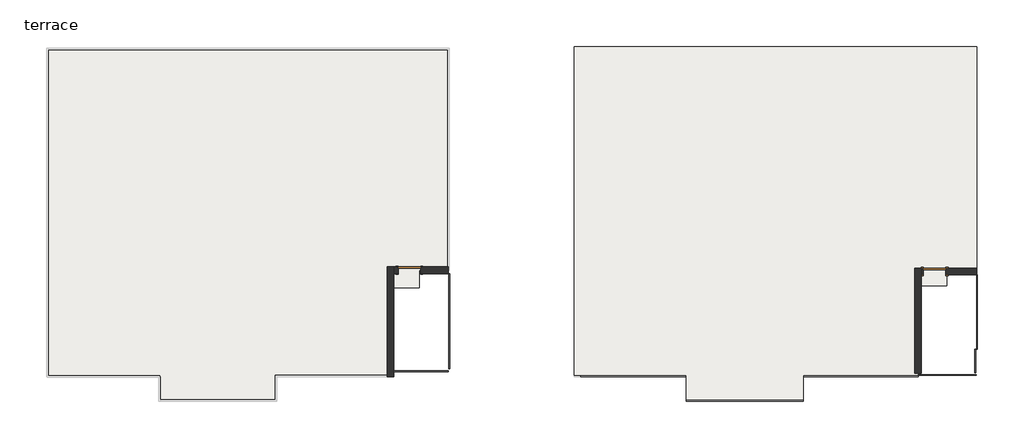
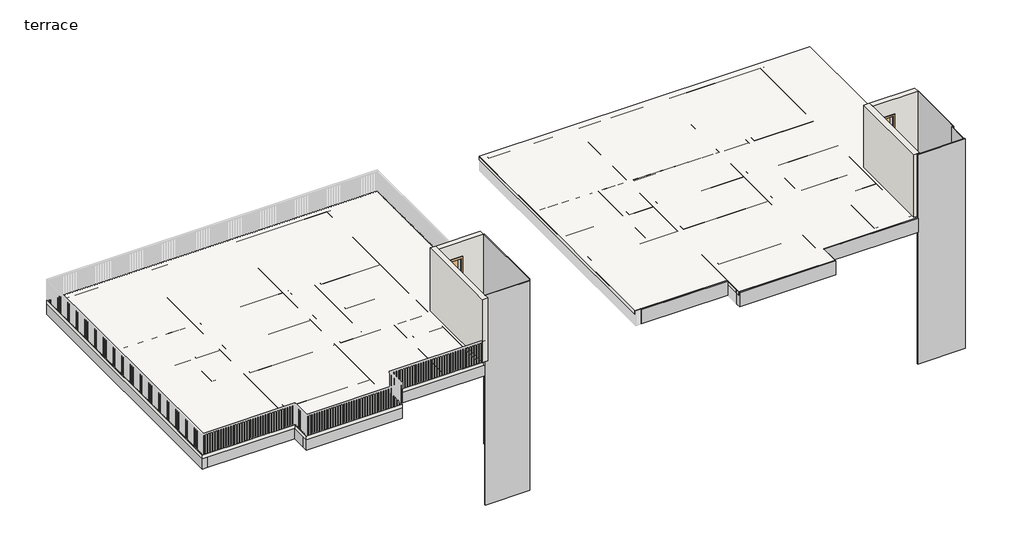
# One storey, part 1 of 6: 27 beams, 5 plates, 4 walls, 2 doors, 2 slabs.
"""IFC4 building model written with IfcOpenShell, lengths in millimetres."""

from ifc_helpers import new_model, si_unit, frame, origin, place, context, project, spatial, polyline, outline, extrude, faceted_brep, transform, mapped, element, save
from components import door_a1484949, system_panel_glazed_3d5b17eb, system_panel_glazed_7e4c53f5, system_panel_glazed_2f845612, system_panel_glazed_6b5749b4, system_panel_glazed_aaff879c

model = new_model("IFC4")

# Units and contexts
model_context = context("Model", 3, world=origin())
ifc_project = project(units=[si_unit("LENGTHUNIT", "METRE", prefix="MILLI")], contexts=[model_context])

# Site, building, storey
site = spatial("IfcSite", under=ifc_project)
building = spatial("IfcBuilding", under=site)
storey = spatial("IfcBuildingStorey", under=building, Name="terrace", Elevation=7010.4)

# Beams
placement = place(None, origin())
element("IfcBeam", 1, ObjectType="Concrete-Rectangular Beam", at=placement, inside=storey, context=model_context, shape_type="Brep", body=[
    faceted_brep([(-16071.9993763, 6519.8935985, 7010.4), (-16300.5993763, 6519.8935985, 7010.4), (-16300.5993763, -4605.3064015, 7010.4), (-16071.9993763, -4605.3064015, 7010.4), (-16071.9993763, -4376.7064015, 7010.4), (-16071.9993763, -1023.9064015, 7010.4), (-16071.9993763, -795.3064015, 7010.4), (-16071.9993763, 728.6935985, 7010.4), (-16071.9993763, 957.2935985, 7010.4), (-16071.9993763, 2592.6672243, 7010.4), (-16071.9993763, 2821.286075, 7010.4), (-16071.9993763, 6291.2935985, 7010.4), (-16300.5993763, 6519.8935985, 6400.8), (-16300.5993763, -4605.3064015, 6400.8), (-16071.9993763, 6519.8935985, 6400.8), (-16071.9993763, 6291.2935985, 6400.8), (-16071.9993763, 2821.286075, 6400.8), (-16071.9993763, 2592.6672243, 6400.8), (-16071.9993763, 957.2935985, 6400.8), (-16071.9993763, 728.6935985, 6400.8), (-16071.9993763, -795.3064015, 6400.8), (-16071.9993763, -1023.9064015, 6400.8), (-16071.9993763, -4376.7064015, 6400.8), (-16071.9993763, -4605.3064015, 6400.8)], [[[0, 1, 2, 3, 4, 5, 6, 7, 8, 9, 10, 11]], [[1, 12, 13, 2]], [[12, 14, 15, 16, 17, 18, 19, 20, 21, 22, 23, 13]], [[14, 0, 11, 10, 9, 8, 7, 6, 5, 4, 3, 23, 22, 21, 20, 19, 18, 17, 16, 15]], [[1, 0, 14, 12]], [[3, 2, 13, 23]]]),
])
element("IfcBeam", 2, ObjectType="Concrete-Rectangular Beam", at=placement, inside=storey, context=model_context, shape_type="SweptSolid", body=[
    extrude(outline(polyline([(-16071.9993763, -4605.3064015), (-16071.9993763, -4376.7064015), (-12490.5993763, -4376.7064015), (-12490.5993763, -4605.3064015), (-16071.9993763, -4605.3064015)])), frame((0.0, 0.0, 6400.8), z_axis=(0.0, 0.0, 1.0), x_axis=(1.0, 0.0, 0.0)), (0.0, 0.0, 1.0), 609.6),
])
element("IfcBeam", 3, ObjectType="Concrete-Rectangular Beam", at=placement, inside=storey, context=model_context, shape_type="Brep", body=[
    faceted_brep([(-8528.1993763, -5443.5064015, 7010.4), (-8528.1993763, -5214.9064015, 7010.4), (-8756.7993763, -5214.9064015, 7010.4), (-12261.9993763, -5214.9064015, 7010.4), (-12490.5993763, -5214.9064015, 7010.4), (-12490.5993763, -5443.5064015, 7010.4), (-8528.1993763, -5443.5064015, 6400.8), (-12490.5993763, -5443.5064015, 6400.8), (-8528.1993763, -5214.9064015, 6400.8), (-12490.5993763, -5214.9064015, 6400.8), (-12261.9993763, -5214.9064015, 6400.8), (-8756.7993763, -5214.9064015, 6400.8)], [[[0, 1, 2, 3, 4, 5]], [[6, 0, 5, 7]], [[8, 6, 7, 9, 10, 11]], [[1, 8, 11, 10, 9, 4, 3, 2]], [[1, 0, 6, 8]], [[5, 4, 9, 7]]]),
])
element("IfcBeam", 4, ObjectType="Concrete-Rectangular Beam", at=placement, inside=storey, context=model_context, shape_type="Brep", body=[
    faceted_brep([(-4641.9993763, 6291.2935985, 7010.4), (-4641.9993763, 6519.8935985, 7010.4), (-16071.9993763, 6519.8935985, 7010.4), (-16071.9993763, 6291.2935985, 7010.4), (-12490.5993763, 6291.2935985, 7010.4), (-12261.9993763, 6291.2935985, 7010.4), (-8756.7993763, 6291.2935985, 7010.4), (-8528.1993763, 6291.2935985, 7010.4), (-4870.5993763, 6291.2935985, 7010.4), (-4641.9993763, 6291.2935985, 6400.8), (-16071.9993763, 6291.2935985, 6400.8), (-12490.5993763, 6291.2935985, 6400.8), (-12261.9993763, 6291.2935985, 6400.8), (-8756.7993763, 6291.2935985, 6400.8), (-8528.1993763, 6291.2935985, 6400.8), (-4870.5993763, 6291.2935985, 6400.8), (-4641.9993763, 6519.8935985, 6400.8), (-16071.9993763, 6519.8935985, 6400.8)], [[[0, 1, 2, 3, 4, 5, 6, 7, 8]], [[9, 0, 8, 7, 6, 5, 4, 3, 10, 11, 12, 13, 14, 15]], [[16, 9, 15, 14, 13, 12, 11, 10, 17]], [[1, 16, 17, 2]], [[3, 2, 17, 10]], [[1, 0, 9, 16]]]),
])
element("IfcBeam", 5, ObjectType="Concrete-Rectangular Beam", at=placement, inside=storey, context=model_context, shape_type="Brep", body=[
    faceted_brep([(-12261.9993763, 6291.2935985, 7010.4), (-12490.5993763, 6291.2935985, 7010.4), (-12490.5993763, 2775.2918938, 7010.4), (-12490.5993763, 2546.6730431, 7010.4), (-12490.5993763, 957.2935985, 7010.4), (-12490.5993763, 728.6935985, 7010.4), (-12490.5993763, -795.3064015, 7010.4), (-12490.5993763, -1023.9064015, 7010.4), (-12490.5993763, -4376.7064015, 7010.4), (-12490.5993763, -4605.3064015, 7010.4), (-12490.5993763, -5214.9064015, 7010.4), (-12261.9993763, -5214.9064015, 7010.4), (-12261.9993763, -3538.5064015, 7010.4), (-12261.9993763, -3309.9064015, 7010.4), (-12261.9993763, -1023.9064015, 7010.4), (-12261.9993763, -795.3064015, 7010.4), (-12261.9993763, 728.6935985, 7010.4), (-12261.9993763, 957.2935985, 7010.4), (-12261.9993763, 2481.2935985, 7010.4), (-12261.9993763, 2709.8935985, 7010.4), (-12261.9993763, 2772.356095, 7010.4), (-12490.5993763, 6291.2935985, 6400.8), (-12490.5993763, 2775.2918938, 6400.8), (-12490.5993763, 2546.6730431, 6400.8), (-12490.5993763, 957.2935985, 6400.8), (-12490.5993763, 728.6935985, 6400.8), (-12490.5993763, -795.3064015, 6400.8), (-12490.5993763, -1023.9064015, 6400.8), (-12490.5993763, -4376.7064015, 6400.8), (-12490.5993763, -4605.3064015, 6400.8), (-12490.5993763, -5214.9064015, 6400.8), (-12261.9993763, 6291.2935985, 6400.8), (-12261.9993763, 2772.356095, 6400.8), (-12261.9993763, 2709.8935985, 6400.8), (-12261.9993763, 2481.2935985, 6400.8), (-12261.9993763, 957.2935985, 6400.8), (-12261.9993763, 728.6935985, 6400.8), (-12261.9993763, -795.3064015, 6400.8), (-12261.9993763, -1023.9064015, 6400.8), (-12261.9993763, -3309.9064015, 6400.8), (-12261.9993763, -3538.5064015, 6400.8), (-12261.9993763, -5214.9064015, 6400.8)], [[[0, 1, 2, 3, 4, 5, 6, 7, 8, 9, 10, 11, 12, 13, 14, 15, 16, 17, 18, 19, 20]], [[1, 21, 22, 23, 24, 25, 26, 27, 28, 29, 30, 10, 9, 8, 7, 6, 5, 4, 3, 2]], [[21, 31, 32, 33, 34, 35, 36, 37, 38, 39, 40, 41, 30, 29, 28, 27, 26, 25, 24, 23, 22]], [[31, 0, 20, 19, 18, 17, 16, 15, 14, 13, 12, 11, 41, 40, 39, 38, 37, 36, 35, 34, 33, 32]], [[1, 0, 31, 21]], [[11, 10, 30, 41]]]),
])
element("IfcBeam", 6, ObjectType="Concrete-Rectangular Beam", at=placement, inside=storey, context=model_context, shape_type="Brep", body=[
    faceted_brep([(-8756.7993763, -5214.9064015, 7010.4), (-8528.1993763, -5214.9064015, 7010.4), (-8528.1993763, -4605.3064015, 7010.4), (-8528.1993763, -4376.7064015, 7010.4), (-8528.1993763, -1023.9064015, 7010.4), (-8528.1993763, -795.3064015, 7010.4), (-8528.1993763, 728.6935985, 7010.4), (-8528.1993763, 957.2935985, 7010.4), (-8528.1993763, 2481.2935985, 7010.4), (-8528.1993763, 2709.8935985, 7010.4), (-8528.1993763, 2724.4047146, 7010.4), (-8528.1993763, 6291.2935985, 7010.4), (-8756.7993763, 6291.2935985, 7010.4), (-8756.7993763, 2727.3405134, 7010.4), (-8756.7993763, 2709.8935985, 7010.4), (-8756.7993763, 2481.2935985, 7010.4), (-8756.7993763, 957.2935985, 7010.4), (-8756.7993763, 728.6935985, 7010.4), (-8756.7993763, -795.3064015, 7010.4), (-8756.7993763, -1023.9064015, 7010.4), (-8756.7993763, -3309.9064015, 7010.4), (-8756.7993763, -3538.5064015, 7010.4), (-8528.1993763, -5214.9064015, 6400.8), (-8528.1993763, -4605.3064015, 6400.8), (-8528.1993763, -4376.7064015, 6400.8), (-8528.1993763, -1023.9064015, 6400.8), (-8528.1993763, -795.3064015, 6400.8), (-8528.1993763, 728.6935985, 6400.8), (-8528.1993763, 957.2935985, 6400.8), (-8528.1993763, 2481.2935985, 6400.8), (-8528.1993763, 2709.8935985, 6400.8), (-8528.1993763, 2724.4047146, 6400.8), (-8528.1993763, 6291.2935985, 6400.8), (-8756.7993763, -5214.9064015, 6400.8), (-8756.7993763, -3538.5064015, 6400.8), (-8756.7993763, -3309.9064015, 6400.8), (-8756.7993763, -1023.9064015, 6400.8), (-8756.7993763, -795.3064015, 6400.8), (-8756.7993763, 728.6935985, 6400.8), (-8756.7993763, 957.2935985, 6400.8), (-8756.7993763, 2481.2935985, 6400.8), (-8756.7993763, 2709.8935985, 6400.8), (-8756.7993763, 2727.3405134, 6400.8), (-8756.7993763, 6291.2935985, 6400.8)], [[[0, 1, 2, 3, 4, 5, 6, 7, 8, 9, 10, 11, 12, 13, 14, 15, 16, 17, 18, 19, 20, 21]], [[1, 22, 23, 24, 25, 26, 27, 28, 29, 30, 31, 32, 11, 10, 9, 8, 7, 6, 5, 4, 3, 2]], [[22, 33, 34, 35, 36, 37, 38, 39, 40, 41, 42, 43, 32, 31, 30, 29, 28, 27, 26, 25, 24, 23]], [[33, 0, 21, 20, 19, 18, 17, 16, 15, 14, 13, 12, 43, 42, 41, 40, 39, 38, 37, 36, 35, 34]], [[1, 0, 33, 22]], [[12, 11, 32, 43]]]),
])
element("IfcBeam", 7, ObjectType="Concrete-Rectangular Beam", at=placement, inside=storey, context=model_context, shape_type="Brep", body=[
    faceted_brep([(-4641.9993763, -4605.3064015, 7010.4), (-4641.9993763, -4376.7064015, 7010.4), (-4870.5993763, -4376.7064015, 7010.4), (-6089.7993763, -4376.7064015, 7010.4), (-6318.3993763, -4376.7064015, 7010.4), (-8528.1993763, -4376.7064015, 7010.4), (-8528.1993763, -4605.3064015, 7010.4), (-4641.9993763, -4376.7064015, 6400.8), (-4870.5993763, -4376.7064015, 6400.8), (-6089.7993763, -4376.7064015, 6400.8), (-6318.3993763, -4376.7064015, 6400.8), (-8528.1993763, -4376.7064015, 6400.8), (-4641.9993763, -4605.3064015, 6400.8), (-8528.1993763, -4605.3064015, 6400.8)], [[[0, 1, 2, 3, 4, 5, 6]], [[1, 7, 8, 9, 10, 11, 5, 4, 3, 2]], [[7, 12, 13, 11, 10, 9, 8]], [[12, 0, 6, 13]], [[6, 5, 11, 13]], [[1, 0, 12, 7]]]),
])
element("IfcBeam", 8, ObjectType="Concrete-Rectangular Beam", at=placement, inside=storey, context=model_context, shape_type="Brep", body=[
    faceted_brep([(-8528.1993763, -795.3064015, 7010.4), (-8528.1993763, -1023.9064015, 7010.4), (-6318.3993763, -1023.9064015, 7010.4), (-6089.7993763, -1023.9064015, 7010.4), (-4870.5993763, -1023.9064015, 7010.4), (-4870.5993763, -795.3064015, 7010.4), (-7308.9993763, -795.3064015, 7010.4), (-7537.5993763, -795.3064015, 7010.4), (-8528.1993763, -795.3064015, 6400.8), (-4870.5993763, -795.3064015, 6400.8), (-7308.9993763, -795.3064015, 6400.8), (-7537.5993763, -795.3064015, 6400.8), (-8528.1993763, -1023.9064015, 6400.8), (-4870.5993763, -1023.9064015, 6400.8), (-6089.7993763, -1023.9064015, 6400.8), (-6318.3993763, -1023.9064015, 6400.8)], [[[0, 1, 2, 3, 4, 5, 6, 7]], [[8, 0, 7, 6, 5, 9, 10, 11]], [[12, 8, 11, 10, 9, 13, 14, 15]], [[1, 12, 15, 14, 13, 4, 3, 2]], [[1, 0, 8, 12]], [[5, 4, 13, 9]]]),
])
element("IfcBeam", 9, ObjectType="Concrete-Rectangular Beam", at=placement, inside=storey, context=model_context, shape_type="Brep", body=[
    faceted_brep([(-6318.3993763, -4376.7064015, 7010.4), (-6089.7993763, -4376.7064015, 7010.4), (-6089.7993763, -2014.5064015, 7010.4), (-6089.7993763, -1785.9064015, 7010.4), (-6089.7993763, -1023.9064015, 7010.4), (-6318.3993763, -1023.9064015, 7010.4), (-6089.7993763, -4376.7064015, 6400.8), (-6089.7993763, -2014.5064015, 6400.8), (-6089.7993763, -1785.9064015, 6400.8), (-6089.7993763, -1023.9064015, 6400.8), (-6318.3993763, -4376.7064015, 6400.8), (-6318.3993763, -1023.9064015, 6400.8)], [[[0, 1, 2, 3, 4, 5]], [[1, 6, 7, 8, 9, 4, 3, 2]], [[6, 10, 11, 9, 8, 7]], [[10, 0, 5, 11]], [[1, 0, 10, 6]], [[5, 4, 9, 11]]]),
])
element("IfcBeam", 10, ObjectType="Concrete-Rectangular Beam", at=placement, inside=storey, context=model_context, shape_type="SweptSolid", body=[
    extrude(outline(polyline([(-4870.5993763, -1785.9064015), (-4870.5993763, -2014.5064015), (-6089.7993763, -2014.5064015), (-6089.7993763, -1785.9064015), (-4870.5993763, -1785.9064015)])), frame((0.0, 0.0, 6400.8), z_axis=(0.0, 0.0, 1.0), x_axis=(1.0, 0.0, 0.0)), (0.0, 0.0, 1.0), 609.6),
])
element("IfcBeam", 11, ObjectType="Concrete-Rectangular Beam", at=placement, inside=storey, context=model_context, shape_type="Brep", body=[
    faceted_brep([(-7308.9993763, 2709.8935985, 7010.4), (-7398.2714156, 2709.8935985, 7010.4), (-7537.5993763, 2709.8935985, 7010.4), (-7537.5993763, 2481.2935985, 7010.4), (-7537.5993763, 957.2935985, 7010.4), (-7537.5993763, 728.6935985, 7010.4), (-7537.5993763, -795.3064015, 7010.4), (-7308.9993763, -795.3064015, 7010.4), (-7308.9993763, 728.6935985, 7010.4), (-7308.9993763, 957.2935985, 7010.4), (-7308.9993763, 2481.2935985, 7010.4), (-7308.9993763, 2709.8935985, 6400.8), (-7308.9993763, -795.3064015, 6400.8), (-7308.9993763, 728.6935985, 6400.8), (-7308.9993763, 957.2935985, 6400.8), (-7308.9993763, 2481.2935985, 6400.8), (-7537.5993763, 2709.8935985, 6400.8), (-7398.2714156, 2709.8935985, 6400.8), (-7537.5993763, -795.3064015, 6400.8), (-7537.5993763, 728.6935985, 6400.8), (-7537.5993763, 957.2935985, 6400.8), (-7537.5993763, 2481.2935985, 6400.8)], [[[0, 1, 2, 3, 4, 5, 6, 7, 8, 9, 10]], [[11, 0, 10, 9, 8, 7, 12, 13, 14, 15]], [[16, 17, 11, 15, 14, 13, 12, 18, 19, 20, 21]], [[2, 16, 21, 20, 19, 18, 6, 5, 4, 3]], [[7, 6, 18, 12]], [[2, 1, 0, 11, 17, 16]]]),
])
element("IfcBeam", 12, ObjectType="Concrete-Rectangular Beam", at=placement, inside=storey, context=model_context, shape_type="SweptSolid", body=[
    extrude(outline(polyline([(-7537.5993763, 2709.8935985), (-7537.5993763, 2481.2935985), (-8528.1993763, 2481.2935985), (-8528.1993763, 2709.8935985), (-7537.5993763, 2709.8935985)])), frame((0.0, 0.0, 6400.8), z_axis=(0.0, 0.0, 1.0), x_axis=(1.0, 0.0, 0.0)), (0.0, 0.0, 1.0), 609.6),
    extrude(outline(polyline([(-12261.9993763, 2481.2935985), (-12261.9993763, 2709.8935985), (-8756.7993763, 2709.8935985), (-8756.7993763, 2481.2935985), (-12261.9993763, 2481.2935985)])), frame((0.0, 0.0, 6400.8), z_axis=(0.0, 0.0, 1.0), x_axis=(1.0, 0.0, 0.0)), (0.0, 0.0, 1.0), 609.6),
])
element("IfcBeam", 13, ObjectType="Concrete-Rectangular Beam", at=placement, inside=storey, context=model_context, shape_type="Brep", body=[
    faceted_brep([(-8756.7993763, -1023.9064015, 7010.4), (-8756.7993763, -795.3064015, 7010.4), (-12261.9993763, -795.3064015, 7010.4), (-12261.9993763, -1023.9064015, 7010.4), (-8756.7993763, -795.3064015, 6400.8), (-12261.9993763, -795.3064015, 6400.8), (-8756.7993763, -1023.9064015, 6400.8), (-12261.9993763, -1023.9064015, 6400.8)], [[[0, 1, 2, 3]], [[1, 4, 5, 2]], [[4, 6, 7, 5]], [[6, 0, 3, 7]], [[1, 0, 6, 4]], [[3, 2, 5, 7]]]),
    faceted_brep([(-16071.9993763, -1023.9064015, 7010.4), (-16071.9993763, -795.3064015, 7010.4), (-16071.9993763, -795.3064015, 6400.8), (-16071.9993763, -1023.9064015, 6400.8), (-12490.5993763, -795.3064015, 7010.4), (-12490.5993763, -1023.9064015, 7010.4), (-12490.5993763, -1023.9064015, 6400.8), (-12490.5993763, -795.3064015, 6400.8), (-13481.1993763, -795.3064015, 7010.4), (-13709.7993763, -795.3064015, 7010.4), (-13481.1993763, -795.3064015, 6400.8), (-13709.7993763, -795.3064015, 6400.8)], [[[0, 1, 2, 3]], [[4, 5, 6, 7]], [[1, 0, 5, 4, 8, 9]], [[2, 1, 9, 8, 4, 7, 10, 11]], [[3, 2, 11, 10, 7, 6]], [[0, 3, 6, 5]]]),
])
element("IfcBeam", 14, ObjectType="Concrete-Rectangular Beam", at=placement, inside=storey, context=model_context, shape_type="Brep", body=[
    faceted_brep([(-13709.7993763, -795.3064015, 7010.4), (-13481.1993763, -795.3064015, 7010.4), (-13481.1993763, 728.6935985, 7010.4), (-13481.1993763, 957.2935985, 7010.4), (-13481.1993763, 2559.3948379, 7010.4), (-13709.7993763, 2562.3306367, 7010.4), (-13709.7993763, 957.2935985, 7010.4), (-13709.7993763, 728.6935985, 7010.4), (-13709.7993763, -795.3064015, 6400.8), (-13709.7993763, 2562.3306367, 6400.8), (-13709.7993763, 957.2935985, 6400.8), (-13709.7993763, 728.6935985, 6400.8), (-13481.1993763, -795.3064015, 6400.8), (-13481.1993763, 2559.3948379, 6400.8), (-13481.1993763, 957.2935985, 6400.8), (-13481.1993763, 728.6935985, 6400.8)], [[[0, 1, 2, 3, 4, 5, 6, 7]], [[8, 0, 7, 6, 5, 9, 10, 11]], [[12, 8, 11, 10, 9, 13, 14, 15]], [[1, 12, 15, 14, 13, 4, 3, 2]], [[1, 0, 8, 12]], [[5, 4, 13, 9]]]),
])
element("IfcBeam", 15, ObjectType="Concrete-Rectangular Beam", at=placement, inside=storey, context=model_context, shape_type="SweptSolid", body=[
    extrude(outline(polyline([(-16071.9993763, 728.6935985), (-16071.9993763, 957.2935985), (-13709.7993763, 957.2935985), (-13709.7993763, 728.6935985), (-16071.9993763, 728.6935985)])), frame((0.0, 0.0, 6400.8), z_axis=(0.0, 0.0, 1.0), x_axis=(1.0, 0.0, 0.0)), (0.0, 0.0, 1.0), 609.6),
])
element("IfcBeam", 16, ObjectType="Concrete-Rectangular Beam", at=placement, inside=storey, context=model_context, shape_type="SweptSolid", body=[
    extrude(outline(polyline([(-12490.5993763, 957.2935985), (-12490.5993763, 728.6935985), (-13481.1993763, 728.6935985), (-13481.1993763, 957.2935985), (-12490.5993763, 957.2935985)])), frame((0.0, 0.0, 6400.8), z_axis=(0.0, 0.0, 1.0), x_axis=(1.0, 0.0, 0.0)), (0.0, 0.0, 1.0), 609.6),
])
element("IfcBeam", 17, ObjectType="Concrete-Rectangular Beam", at=placement, inside=storey, context=model_context, shape_type="SweptSolid", body=[
    extrude(outline(polyline([(-12261.9993763, 728.6935985), (-12261.9993763, 957.2935985), (-8756.7993763, 957.2935985), (-8756.7993763, 728.6935985), (-12261.9993763, 728.6935985)])), frame((0.0, 0.0, 6400.8), z_axis=(0.0, 0.0, 1.0), x_axis=(1.0, 0.0, 0.0)), (0.0, 0.0, 1.0), 609.6),
    extrude(outline(polyline([(-7537.5993763, 957.2935985), (-7537.5993763, 728.6935985), (-8528.1993763, 728.6935985), (-8528.1993763, 957.2935985), (-7537.5993763, 957.2935985)])), frame((0.0, 0.0, 6400.8), z_axis=(0.0, 0.0, 1.0), x_axis=(1.0, 0.0, 0.0)), (0.0, 0.0, 1.0), 609.6),
])
element("IfcBeam", 18, ObjectType="Concrete-Rectangular Beam", at=placement, inside=storey, context=model_context, shape_type="Brep", body=[
    faceted_brep([(-12490.5993763, 2546.6730431, 7010.4), (-12490.5993763, 2775.2918938, 7010.4), (-16071.9993763, 2821.286075, 7010.4), (-16071.9993763, 2592.6672243, 7010.4), (-13709.7993763, 2562.3306367, 7010.4), (-13481.1993763, 2559.3948379, 7010.4), (-12490.5993763, 2775.2918938, 6400.8), (-16071.9993763, 2821.286075, 6400.8), (-12490.5993763, 2546.6730431, 6400.8), (-13481.1993763, 2559.3948379, 6400.8), (-13709.7993763, 2562.3306367, 6400.8), (-16071.9993763, 2592.6672243, 6400.8)], [[[0, 1, 2, 3, 4, 5]], [[1, 6, 7, 2]], [[6, 8, 9, 10, 11, 7]], [[8, 0, 5, 4, 3, 11, 10, 9]], [[6, 1, 0, 8]], [[3, 2, 7, 11]]]),
    faceted_brep([(-12261.9993763, 2709.8935985, 7010.4), (-12261.9993763, 2709.8935985, 6400.8), (-8756.7993763, 2709.8935985, 6400.8), (-8756.7993763, 2709.8935985, 7010.4), (-12261.9993763, 2772.356095, 7010.4), (-12261.9993763, 2772.356095, 6400.8), (-8756.7993763, 2727.3405134, 7010.4), (-8756.7993763, 2727.3405134, 6400.8)], [[[0, 1, 2, 3]], [[0, 4, 5, 1]], [[4, 0, 3, 6]], [[5, 4, 6, 7]], [[1, 5, 7, 2]], [[3, 2, 7, 6]]]),
    faceted_brep([(-8528.1993763, 2709.8935985, 6400.8), (-8528.1993763, 2709.8935985, 7010.4), (-8528.1993763, 2724.4047146, 7010.4), (-8528.1993763, 2724.4047146, 6400.8), (-7398.2714156, 2709.8935985, 6400.8), (-7398.2714156, 2709.8935985, 7010.4), (-7537.5993763, 2709.8935985, 7010.4), (-7537.5993763, 2709.8935985, 6400.8)], [[[0, 1, 2, 3]], [[4, 5, 6, 1, 0, 7]], [[1, 6, 5, 2]], [[5, 4, 3, 2]], [[4, 7, 0, 3]]]),
])
element("IfcBeam", 19, ObjectType="Concrete-Rectangular Beam", at=placement, inside=storey, context=model_context, shape_type="SweptSolid", body=[
    extrude(outline(polyline([(-12261.9993763, -3538.5064015), (-12261.9993763, -3309.9064015), (-8756.7993763, -3309.9064015), (-8756.7993763, -3538.5064015), (-12261.9993763, -3538.5064015)])), frame((0.0, 0.0, 6400.8), z_axis=(0.0, 0.0, 1.0), x_axis=(1.0, 0.0, 0.0)), (0.0, 0.0, 1.0), 609.6),
])
element("IfcBeam", 20, ObjectType="Concrete-Rectangular Beam", at=placement, inside=storey, context=model_context, shape_type="SweptSolid", body=[
    extrude(outline(polyline([(1802.5761273, -4605.3064015), (1802.5761273, -4376.7064015), (5383.9761273, -4376.7064015), (5383.9761273, -4605.3064015), (1802.5761273, -4605.3064015)])), frame((0.0, 0.0, 6400.8), z_axis=(0.0, 0.0, 1.0), x_axis=(1.0, 0.0, 0.0)), (0.0, 0.0, 1.0), 609.6),
])
element("IfcBeam", 21, ObjectType="Concrete-Rectangular Beam", at=placement, inside=storey, context=model_context, shape_type="Brep", body=[
    faceted_brep([(9346.3761273, -5443.5064015, 7010.4), (9346.3761273, -5214.9064015, 7010.4), (9117.7761273, -5214.9064015, 7010.4), (5612.5761273, -5214.9064015, 7010.4), (5383.9761273, -5214.9064015, 7010.4), (5383.9761273, -5443.5064015, 7010.4), (9346.3761273, -5443.5064015, 6400.8), (5383.9761273, -5443.5064015, 6400.8), (9346.3761273, -5214.9064015, 6400.8), (5383.9761273, -5214.9064015, 6400.8), (5612.5761273, -5214.9064015, 6400.8), (9117.7761273, -5214.9064015, 6400.8)], [[[0, 1, 2, 3, 4, 5]], [[6, 0, 5, 7]], [[8, 6, 7, 9, 10, 11]], [[1, 8, 11, 10, 9, 4, 3, 2]], [[1, 0, 6, 8]], [[5, 4, 9, 7]]]),
])
element("IfcBeam", 22, ObjectType="Concrete-Rectangular Beam", at=placement, inside=storey, context=model_context, shape_type="Brep", body=[
    faceted_brep([(13232.5761273, -4605.3064015, 7010.4), (13232.5761273, -4376.7064015, 7010.4), (13003.9761273, -4376.7064015, 7010.4), (11784.7761273, -4376.7064015, 7010.4), (11556.1761273, -4376.7064015, 7010.4), (9346.3761273, -4376.7064015, 7010.4), (9346.3761273, -4605.3064015, 7010.4), (13232.5761273, -4376.7064015, 6400.8), (13003.9761273, -4376.7064015, 6400.8), (11784.7761273, -4376.7064015, 6400.8), (11556.1761273, -4376.7064015, 6400.8), (9346.3761273, -4376.7064015, 6400.8), (13232.5761273, -4605.3064015, 6400.8), (9346.3761273, -4605.3064015, 6400.8)], [[[0, 1, 2, 3, 4, 5, 6]], [[1, 7, 8, 9, 10, 11, 5, 4, 3, 2]], [[7, 12, 13, 11, 10, 9, 8]], [[12, 0, 6, 13]], [[6, 5, 11, 13]], [[1, 0, 12, 7]]]),
])
element("IfcBeam", 23, ObjectType="Concrete-Rectangular Beam", at=placement, inside=storey, context=model_context, shape_type="Brep", body=[
    faceted_brep([(9346.3761273, -795.3064015, 7010.4), (9346.3761273, -1023.9064015, 7010.4), (11556.1761273, -1023.9064015, 7010.4), (11784.7761273, -1023.9064015, 7010.4), (13003.9761273, -1023.9064015, 7010.4), (13003.9761273, -795.3064015, 7010.4), (10565.5761273, -795.3064015, 7010.4), (10336.9761273, -795.3064015, 7010.4), (9346.3761273, -795.3064015, 6400.8), (13003.9761273, -795.3064015, 6400.8), (10565.5761273, -795.3064015, 6400.8), (10336.9761273, -795.3064015, 6400.8), (9346.3761273, -1023.9064015, 6400.8), (13003.9761273, -1023.9064015, 6400.8), (11784.7761273, -1023.9064015, 6400.8), (11556.1761273, -1023.9064015, 6400.8)], [[[0, 1, 2, 3, 4, 5, 6, 7]], [[8, 0, 7, 6, 5, 9, 10, 11]], [[12, 8, 11, 10, 9, 13, 14, 15]], [[1, 12, 15, 14, 13, 4, 3, 2]], [[1, 0, 8, 12]], [[5, 4, 13, 9]]]),
])
element("IfcBeam", 24, ObjectType="Concrete-Rectangular Beam", at=placement, inside=storey, context=model_context, shape_type="Brep", body=[
    faceted_brep([(11556.1761273, -4376.7064015, 7010.4), (11784.7761273, -4376.7064015, 7010.4), (11784.7761273, -2014.5064015, 7010.4), (11784.7761273, -1785.9064015, 7010.4), (11784.7761273, -1023.9064015, 7010.4), (11556.1761273, -1023.9064015, 7010.4), (11784.7761273, -4376.7064015, 6400.8), (11784.7761273, -2014.5064015, 6400.8), (11784.7761273, -1785.9064015, 6400.8), (11784.7761273, -1023.9064015, 6400.8), (11556.1761273, -4376.7064015, 6400.8), (11556.1761273, -1023.9064015, 6400.8)], [[[0, 1, 2, 3, 4, 5]], [[1, 6, 7, 8, 9, 4, 3, 2]], [[6, 10, 11, 9, 8, 7]], [[10, 0, 5, 11]], [[1, 0, 10, 6]], [[5, 4, 9, 11]]]),
])
element("IfcBeam", 25, ObjectType="Concrete-Rectangular Beam", at=placement, inside=storey, context=model_context, shape_type="SweptSolid", body=[
    extrude(outline(polyline([(13003.9761273, -1785.9064015), (13003.9761273, -2014.5064015), (11784.7761273, -2014.5064015), (11784.7761273, -1785.9064015), (13003.9761273, -1785.9064015)])), frame((0.0, 0.0, 6400.8), z_axis=(0.0, 0.0, 1.0), x_axis=(1.0, 0.0, 0.0)), (0.0, 0.0, 1.0), 609.6),
])
element("IfcBeam", 26, ObjectType="Concrete-Rectangular Beam", at=placement, inside=storey, context=model_context, shape_type="Brep", body=[
    faceted_brep([(9117.7761273, -1023.9064015, 7010.4), (9117.7761273, -795.3064015, 7010.4), (5612.5761273, -795.3064015, 7010.4), (5612.5761273, -1023.9064015, 7010.4), (9117.7761273, -795.3064015, 6400.8), (5612.5761273, -795.3064015, 6400.8), (9117.7761273, -1023.9064015, 6400.8), (5612.5761273, -1023.9064015, 6400.8)], [[[0, 1, 2, 3]], [[1, 4, 5, 2]], [[4, 6, 7, 5]], [[6, 0, 3, 7]], [[1, 0, 6, 4]], [[3, 2, 5, 7]]]),
    faceted_brep([(1802.5761273, -1023.9064015, 7010.4), (1802.5761273, -795.3064015, 7010.4), (1802.5761273, -795.3064015, 6400.8), (1802.5761273, -1023.9064015, 6400.8), (5383.9761273, -795.3064015, 7010.4), (5383.9761273, -1023.9064015, 7010.4), (5383.9761273, -1023.9064015, 6400.8), (5383.9761273, -795.3064015, 6400.8), (4393.3761273, -795.3064015, 7010.4), (4164.7761273, -795.3064015, 7010.4), (4393.3761273, -795.3064015, 6400.8), (4164.7761273, -795.3064015, 6400.8)], [[[0, 1, 2, 3]], [[4, 5, 6, 7]], [[1, 0, 5, 4, 8, 9]], [[2, 1, 9, 8, 4, 7, 10, 11]], [[3, 2, 11, 10, 7, 6]], [[0, 3, 6, 5]]]),
])
element("IfcBeam", 27, ObjectType="Concrete-Rectangular Beam", at=placement, inside=storey, context=model_context, shape_type="SweptSolid", body=[
    extrude(outline(polyline([(5612.5761273, -3538.5064015), (5612.5761273, -3309.9064015), (9117.7761273, -3309.9064015), (9117.7761273, -3538.5064015), (5612.5761273, -3538.5064015)])), frame((0.0, 0.0, 6400.8), z_axis=(0.0, 0.0, 1.0), x_axis=(1.0, 0.0, 0.0)), (0.0, 0.0, 1.0), 609.6),
])

# Doors
door_shape = door_a1484949(model_context)
element("IfcDoor", 28, ObjectType="Single-Flush : 30\" x 80\"", at=placement, inside=storey, context=model_context, shape_type="MappedRepresentation", body=[
    mapped(door_shape, transform((-4006.9993763, -998.5064015, 7010.4), x_axis=(1.0, 0.0, 0.0), y_axis=(0.0, 1.0, 0.0), z_axis=(0.0, 0.0, 1.0))),
])
element("IfcDoor", 29, ObjectType="Single-Flush : 30\" x 80\"", at=placement, inside=storey, context=model_context, shape_type="MappedRepresentation", body=[
    mapped(door_shape, transform((13791.3761273, -1042.9564015, 7010.4), x_axis=(1.0, 0.0, 0.0), y_axis=(0.0, 1.0, 0.0), z_axis=(0.0, 0.0, 1.0))),
])

# Plates
system_panel_glazed_shape = system_panel_glazed_3d5b17eb(model_context)
element("IfcPlate", 30, ObjectType="System Panel : Glazed", at=placement, inside=storey, context=model_context, shape_type="MappedRepresentation", body=[
    mapped(system_panel_glazed_shape, transform((15201.7506237, -2416.6158957, 609.6), x_axis=(0.0, -1.0, 0.0), y_axis=(1.0, 0.0, 0.0), z_axis=(0.0, 0.0, 1.0))),
])
system_panel_glazed_2_shape = system_panel_glazed_7e4c53f5(model_context)
element("IfcPlate", 31, ObjectType="System Panel : Glazed", at=placement, inside=storey, context=model_context, shape_type="MappedRepresentation", body=[
    mapped(system_panel_glazed_2_shape, transform((15201.7506237, -4070.7908957, 609.6), x_axis=(0.0, 1.0, 0.0), y_axis=(-1.0, 0.0, 0.0), z_axis=(0.0, 0.0, 1.0))),
])
system_panel_glazed_3_shape = system_panel_glazed_2f845612(model_context)
element("IfcPlate", 32, ObjectType="System Panel : Glazed", at=placement, inside=storey, context=model_context, shape_type="MappedRepresentation", body=[
    mapped(system_panel_glazed_3_shape, transform((14217.1633755, -4579.9064015, 609.6), x_axis=(1.0, 0.0, 0.0), y_axis=(0.0, 1.0, 0.0), z_axis=(0.0, 0.0, 1.0))),
])
system_panel_glazed_4_shape = system_panel_glazed_6b5749b4(model_context)
element("IfcPlate", 33, ObjectType="System Panel : Glazed", at=placement, inside=storey, context=model_context, shape_type="MappedRepresentation", body=[
    mapped(system_panel_glazed_4_shape, transform((-2686.1993763, -2725.7064015, 609.6), x_axis=(0.0, -1.0, 0.0), y_axis=(1.0, 0.0, 0.0), z_axis=(0.0, 0.0, 1.0))),
])
system_panel_glazed_5_shape = system_panel_glazed_aaff879c(model_context)
element("IfcPlate", 34, ObjectType="System Panel : Glazed", at=placement, inside=storey, context=model_context, shape_type="MappedRepresentation", body=[
    mapped(system_panel_glazed_5_shape, transform((-3606.9493763, -4452.9064015, 609.6), x_axis=(1.0, 0.0, 0.0), y_axis=(0.0, 1.0, 0.0), z_axis=(0.0, 0.0, 1.0))),
])

# Slabs
element("IfcSlab", 35, at=placement, inside=storey, context=model_context, shape_type="SweptSolid", body=[
    extrude(outline(polyline([(-2647.3594779, 6526.2435985), (-2647.3594779, -998.5064015), (-3676.7993763, -998.5064015), (-3676.7993763, -1582.7064015), (-4641.9993763, -1582.7064015), (-4641.9993763, -4605.3064015), (-4692.7993763, -4605.3064015), (-8528.1993763, -4605.3064015), (-8528.1993763, -5443.5064015), (-12490.5993763, -5443.5064015), (-12490.5993763, -4611.6564015), (-16300.5993763, -4611.6564015), (-16300.5993763, 6526.2435985), (-2647.3594779, 6526.2435985)])), frame((0.0, 0.0, 6858.0), z_axis=(0.0, 0.0, 1.0), x_axis=(1.0, 0.0, 0.0)), (0.0, 0.0, 1.0), 152.4),
])
element("IfcSlab", 36, at=placement, inside=storey, context=model_context, shape_type="SweptSolid", body=[
    extrude(outline(polyline([(15227.2160257, 6583.3935985), (15227.2160257, -1042.9564015), (14197.7761273, -1042.9564015), (14197.7761273, -1525.5564015), (13232.5761273, -1525.5564015), (13232.5761273, -4548.1564015), (13181.7761273, -4548.1564015), (9346.3761273, -4548.1564015), (9346.3761273, -5386.3564015), (5383.9761273, -5386.3564015), (5383.9761273, -4554.5064015), (1573.9761273, -4554.5064015), (1573.9761273, 6583.3935985), (15227.2160257, 6583.3935985)])), frame((0.0, 0.0, 6858.0), z_axis=(0.0, 0.0, 1.0), x_axis=(1.0, 0.0, 0.0)), (0.0, 0.0, 1.0), 152.4),
])

# Walls
element("IfcWall", 37, at=placement, inside=storey, context=model_context, shape_type="Brep", body=[
    faceted_brep([(-4527.6993763, -4605.3064015, 7010.4), (-4527.6993763, -4567.2064015, 7010.4), (-4527.6993763, -4338.6064015, 7010.4), (-4527.6993763, -1112.8064015, 7010.4), (-4527.6993763, -884.2064015, 7010.4), (-4527.6993763, -884.2064015, 9753.6), (-4527.6993763, -1112.8064015, 9753.6), (-4527.6993763, -4338.6064015, 9753.6), (-4527.6993763, -4567.2064015, 9753.6), (-4527.6993763, -4605.3064015, 9753.6), (-4756.2993763, -4605.3064015, 7010.4), (-4756.2993763, -4605.3064015, 9753.6), (-4756.2993763, -884.2064015, 9753.6), (-4756.2993763, -884.2064015, 7010.4)], [[[0, 1, 2, 3, 4, 5, 6, 7, 8, 9]], [[10, 11, 12, 13]], [[4, 3, 2, 1, 0, 10, 13]], [[9, 8, 7, 6, 5, 12, 11]], [[0, 9, 11, 10]], [[5, 4, 13, 12]]]),
])
element("IfcWall", 38, at=placement, inside=storey, context=model_context, shape_type="SweptSolid", body=[
    extrude(outline(polyline([(9042.4, -3625.9993763), (7010.4, -3625.9993763), (7010.4, -2686.1993763), (9753.6, -2686.1993763), (9753.6, -4527.6993763), (7010.4, -4527.6993763), (7010.4, -4387.9993763), (9042.4, -4387.9993763), (9042.4, -3625.9993763)])), frame((0.0, -1112.8064015, 0.0), z_axis=(0.0, 1.0, 0.0), x_axis=(0.0, 0.0, 1.0)), (0.0, 0.0, 1.0), 228.6),
])
element("IfcWall", 39, at=placement, inside=storey, context=model_context, shape_type="Brep", body=[
    faceted_brep([(13346.8761273, -4491.0064015, 7010.4), (13346.8761273, -1157.2564015, 7010.4), (13346.8761273, -928.6564015, 7010.4), (13346.8761273, -928.6564015, 9753.6), (13346.8761273, -1157.2564015, 9753.6), (13346.8761273, -4491.0064015, 9753.6), (13118.2761273, -4491.0064015, 7010.4), (13118.2761273, -4491.0064015, 9753.6), (13118.2761273, -928.6564015, 9753.6), (13118.2761273, -928.6564015, 7010.4)], [[[0, 1, 2, 3, 4, 5]], [[6, 7, 8, 9]], [[2, 1, 0, 6, 9]], [[5, 4, 3, 8, 7]], [[0, 5, 7, 6]], [[3, 2, 9, 8]]]),
])
element("IfcWall", 40, at=placement, inside=storey, context=model_context, shape_type="SweptSolid", body=[
    extrude(outline(polyline([(7010.4, 15217.6910257), (9753.6, 15217.6910257), (9753.6, 13346.8761273), (7010.4, 13346.8761273), (7010.4, 13410.3761273), (9042.4, 13410.3761273), (9042.4, 14172.3761273), (7010.4, 14172.3761273), (7010.4, 15217.6910257)])), frame((0.0, -1157.2564015, 0.0), z_axis=(0.0, 1.0, 0.0), x_axis=(0.0, 0.0, 1.0)), (0.0, 0.0, 1.0), 228.6),
])

save(model, "model.ifc")

# Revit data of these elements
# Type "Concrete-Rectangular Beam"
#   Assembly Code = "B10"
#   Length [instance default] = 5' - 0"
#   b = 0' - 9"
#   h = 2' - 0"
#   Structural Material [instance default] = Concrete, Cast-in-Place gray
# Type "Single-Flush : 30\" x 80\""
#   Type Mark = "5"
#   Construction Type Id = "MDOOR"
#   Assembly Code = "C1020"
#   Analytic Construction = "Metal"
#   Thickness = 0' - 2"
#   Heat Transfer Coefficient (U) = 0.651978 BTU/(h·ft²·°F)
#   Height = 6' - 8"
#   Trim Projection Ext = 0' - 1"
#   Trim Projection Int = 0' - 1"
#   Trim Width = 0' - 3"
#   Width = 2' - 6"
#   Define Thermal Properties by = 1
#   Define Thermal Properties by = 1
#   Door Material = Door - Panel
#   Frame Material = Door - Frame
#   Visual Light Transmittance = 0
#   Solar Heat Gain Coefficient = 0
#   Function = (empty or 0)
#   Wall Closure = (empty or 0)
# Type "System Panel : Glazed"
#   Construction Type Id = "GSP4R"
#   Analytic Construction = "1/8 in Pilkington single glazing"
#   Visual Light Transmittance = 0.9
#   Solar Heat Gain Coefficient = 0.86
#   Heat Transfer Coefficient (U) = 1.18115 BTU/(h·ft²·°F)
#   Define Thermal Properties by = 1
# Type
#   Assembly Code = "B1010"
#   Function = 0
#   Layers, outside or top first: 0' - 6" "Concrete, Cast-in-Place gray" (function 1)
# Type
#   Assembly Code = "B2010"
#   Layers, outside or top first: 0' - 9" no material (function 1)
# Elements 1, 2, 3, 4, 5, 6, 7, 8, 9, 10, 11, 12, 13, 14, 15, 16, 17, 18, 19, 20, 21, 22, 23, 24, 25, 26, 27 (IfcBeam, "Concrete-Rectangular Beam")
#   Structural Material = Concrete, Cast-in-Place gray
#   Phase Created = New Construction
#   Materials on its faces: "Concrete, Cast-in-Place gray"
# Elements 28, 29 (IfcDoor, "Single-Flush : 30\" x 80\"")
#   Phase Created = New Construction
#   Materials on its faces: "Door - Frame", "Door - Panel"
# Elements 30, 31, 32, 33, 34 (IfcPlate, "System Panel : Glazed")
#   Phase Created = New Construction
#   Materials on its faces: "Glass"
# Elements 35, 36 (IfcSlab)
#   Height Offset From Level = 0' - 0"
#   Phase Created = New Construction
#   Materials on its faces: "Concrete, Cast-in-Place gray"
# Elements 37, 38, 39, 40 (IfcWall)
#   Top Offset = 0' - 0"
#   Base Offset = 0' - 0"
#   wall height = 9' - 0"
#   Phase Created = New Construction
#   Base Constraint = terrace
#   Top Constraint = staircase head room
#   Materials on its faces: "Default Wall"
# Materials
#   "Concrete, Cast-in-Place gray": class "Concrete", colour RGB 192 192 192, transparency 0, Description = "Cast-in-place concrete", Cost = 0
#   "Door - Panel": class "Wood", colour RGB 210 159 95, transparency 0, Cost = 0
#   "Door - Frame": colour RGB 118 70 51, transparency 0, Cost = 0
#   "Glass": class "Glass", colour RGB 0 128 192, transparency 0.75, Description = "Soda Lime Glass", Cost = 0
#   "Default Wall": colour RGB 128 128 128, transparency 0, Cost = 0
